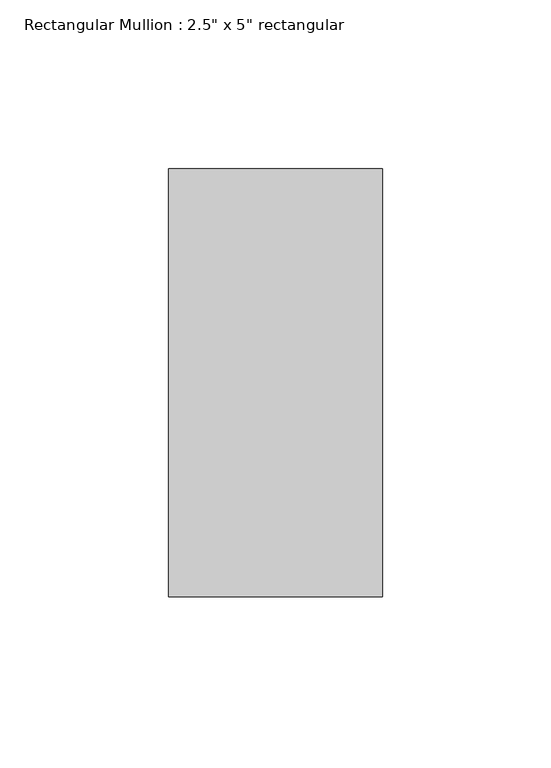
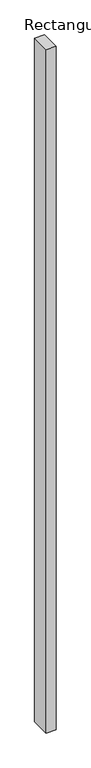
"""IFC4 building model written with IfcOpenShell, lengths in millimetres: member geometry."""

from ifc_helpers import new_model, si_unit, frame, origin, place, context, project, spatial, polyline, outline, extrude, source, transform, mapped, element, save


def member_2afbfae4(model_context):
    return source(origin(), model_context, "Body", "SweptSolid", [
        extrude(outline(polyline([(0.0, 63.5), (0.0, -63.5), (-63.5, -63.5), (-63.5, 63.5), (0.0, 63.5)])), frame((0.0, 0.0, -4605.1256222), z_axis=(0.0, 0.0, 1.0), x_axis=(1.0, 0.0, 0.0)), (0.0, 0.0, 1.0), 4605.1256222),
    ])


if __name__ == "__main__":
    model = new_model("IFC4")
    model_context = context("Model", 3, world=origin())
    ifc_project = project(units=[si_unit("LENGTHUNIT", "METRE", prefix="MILLI")], contexts=[model_context])
    site = spatial("IfcSite", under=ifc_project)
    building = spatial("IfcBuilding", under=site)
    placement = place(None, origin())
    member_shape = member_2afbfae4(model_context)
    element("IfcMember", 1, ObjectType="Rectangular Mullion : 2.5\" x 5\" rectangular", at=placement, inside=building, context=model_context, shape_type="MappedRepresentation", body=[
        mapped(member_shape, transform((0.0, 0.0, 0.0), x_axis=(1.0, 0.0, 0.0), y_axis=(0.0, 1.0, 0.0), z_axis=(0.0, 0.0, 1.0))),
    ])
    save(model, "model.ifc")

# Revit data of these elements
# Type "Rectangular Mullion : 2.5\" x 5\" rectangular"
#   built-in parameter 1007304 = 0.416667 (stored number, unit not read)
#   built-in parameter 1007301 = 0.104167 (stored number, unit not read)
#   built-in parameter 1007300 = 0.104167 (stored number, unit not read)
# Element 1 (IfcMember, "Rectangular Mullion : 2.5\" x 5\" rectangular")
#   Materials on its faces: "Aluminum"
# Materials
#   "Aluminum": class "Metal", colour RGB 247 247 247, transparency 0, Description = "Aluminum 6061", Cost = 0
